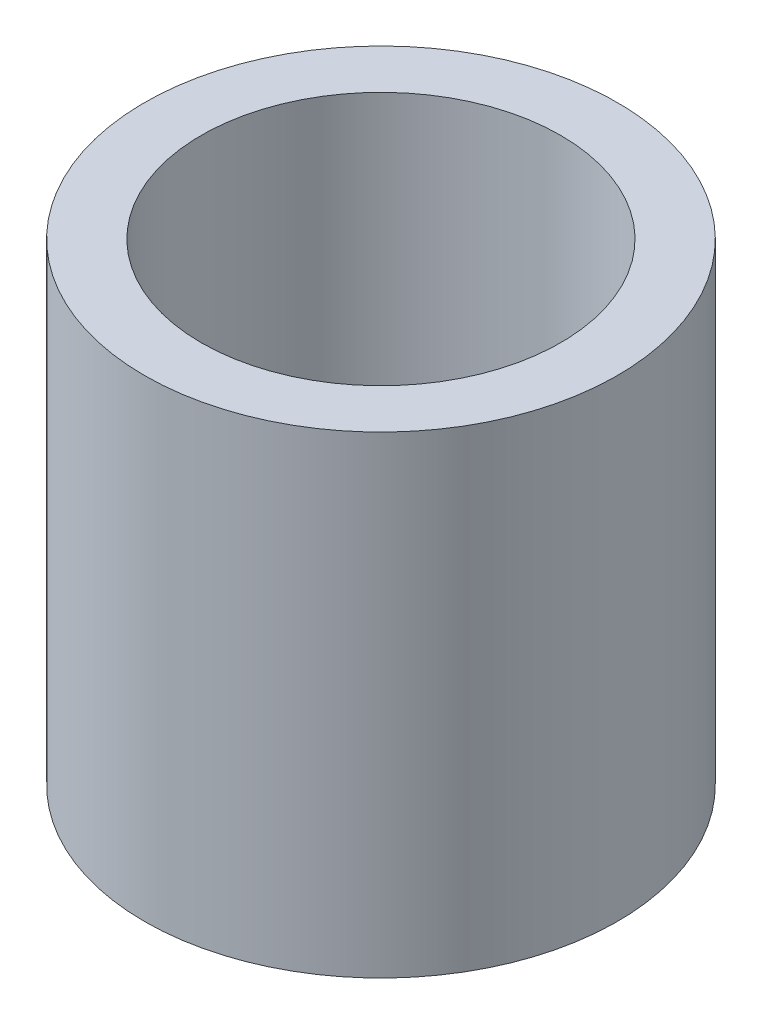
SolidWorks part; units mm, degrees
material "Plain Carbon Steel"
ref_plane "Front Plane" through (0, 0, 0) normal (0, 0, 1) x (1, 0, 0)
ref_plane "Top Plane" through (0, 0, 0) normal (0, 1, 0) x (1, 0, 0)
ref_plane "Right Plane" through (0, 0, 0) normal (1, 0, 0) x (0, 0, -1)
sketch "Bushing Profile Ø25xØ19" plane through (0, 0, 0) normal (0, 1, 0) x (1, 0, 0)
  circle A0 centre (0, 0) radius 12.5
  circle A1 centre (0, 0) radius 9.5
  dimension "D1" = 25
  dimension "D2" = 19
extrude "Bushing Body L25" add sketch "Bushing Profile Ø25xØ19" along normal blind 25
